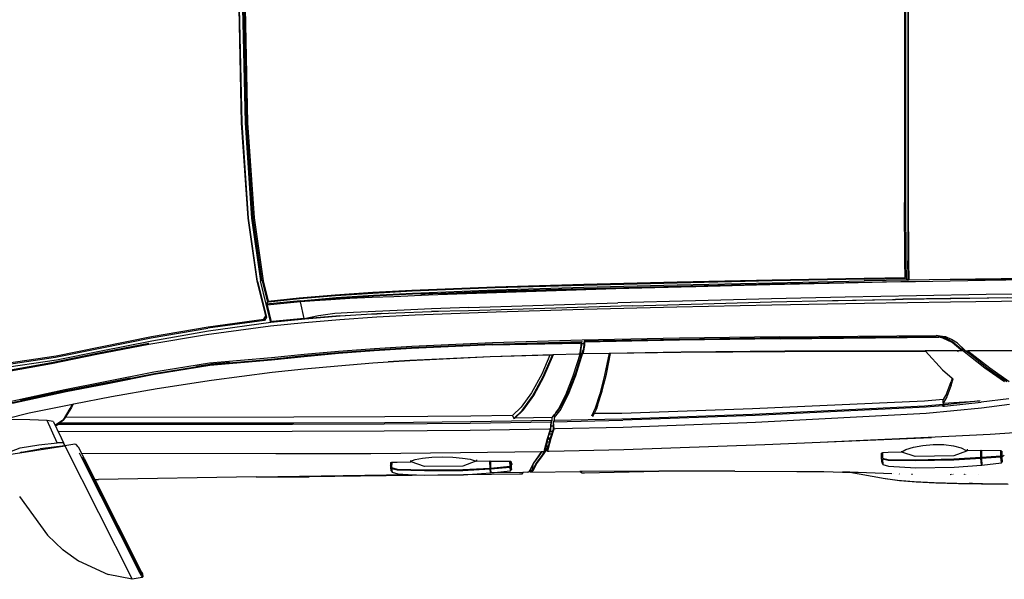
# Model space of a CAD drawing. Units: inches. Extents: x 22042254 to 25404563, y 17568978 to 17626777.
# Tile 5 of 45: x 22042255.014 to 22042256.16, y 17568977.553 to 17568978.204. Entities that reach past the tile are written whole.
import ezdxf

# ---------------------------------------------------------------- set-up
doc = ezdxf.new("R2010")
doc.units = ezdxf.units.IN
doc.header["$MEASUREMENT"] = 0
doc.layers.add('A-SITE-VEHI', color=8, linetype='Continuous', lineweight=18)
doc.layers.add('Edges', color=250, linetype='Continuous')

# ---------------------------------------------------------------- blocks, each defined once
blk = doc.blocks.new('Nissan Qashqai pl')
at = {"layer": 'Edges'}
for p, q in [((8.8918, 12.7444), (9.0186, 12.9956)), ((9.0186, 12.9956), (8.9731, 12.9865)), ((9.0374, 12.9925), (9.0186, 12.9956)), ((8.9173, 12.961), (8.9731, 12.9865)), ((9.0333, 12.9845), (8.9232, 12.7662)), ((9.0386, 12.9907), (8.9254, 12.7664)), ((8.9483, 12.8082), (9.0343, 12.9785)), ((9.0356, 12.9888), (9.0333, 12.9845)), ((9.0343, 12.9785), (9.0347, 12.9794)), ((9.0347, 12.9794), (9.0362, 12.9822)), ((9.0356, 12.9888), (9.0374, 12.9925)), ((9.0362, 12.9822), (9.037, 12.9838)), ((9.0371, 12.9841), (9.037, 12.9838)), ((9.0371, 12.9841), (9.0376, 12.985)), ((9.0376, 12.985), (9.0371, 12.9847)), ((9.0386, 12.9907), (9.0374, 12.9925)), ((9.0376, 12.985), (9.0386, 12.9907)), ((8.8885, 12.9405), (8.9173, 12.961)), ((8.8591, 12.9127), (8.8879, 12.94)), ((8.8885, 12.9405), (8.8879, 12.94)), ((8.8066, 12.84), (8.8591, 12.9127)), ((10.4573, 12.8093), (10.4889, 12.8119)), ((10.4613, 12.8099), (10.4926, 12.8125)), ((10.4889, 12.8119), (10.526, 12.8138)), ((10.4926, 12.8125), (10.5294, 12.8143)), ((10.526, 12.8138), (10.569, 12.8151)), ((10.5294, 12.8143), (10.5719, 12.8156)), ((10.569, 12.8151), (10.5919, 12.8155)), ((10.5719, 12.8156), (10.6176, 12.8164)), ((10.5919, 12.8155), (10.6151, 12.8159)), ((10.5981, 12.8157), (10.5919, 12.8155)), ((10.6174, 12.816), (10.5981, 12.8157)), ((10.6151, 12.8159), (10.6644, 12.8162)), ((10.6176, 12.8164), (10.6651, 12.8167)), ((8.928, 12.7679), (8.9483, 12.8082)), ((8.9483, 12.8082), (8.9552, 12.8081)), ((9.2517, 12.8031), (8.9552, 12.8081)), ((9.2517, 12.8031), (9.351, 12.803)), ((9.2517, 12.8031), (9.5372, 12.7983)), ((9.641, 12.7991), (9.351, 12.803)), ((9.5052, 12.7918), (9.5044, 12.7856)), ((9.5052, 12.7918), (9.5069, 12.7941)), ((9.5061, 12.7878), (9.5069, 12.7941)), ((9.5069, 12.7941), (9.5176, 12.7972)), ((9.5679, 12.792), (9.5168, 12.7904)), ((9.5176, 12.7972), (9.5372, 12.7983)), ((9.5372, 12.7983), (9.5689, 12.7999)), ((9.6401, 12.7914), (9.5679, 12.792)), ((9.5689, 12.7999), (9.641, 12.7991)), ((9.641, 12.7991), (9.6921, 12.7956)), ((9.7466, 12.7978), (9.641, 12.7991)), ((9.692, 12.7943), (9.6913, 12.7886)), ((9.6921, 12.7956), (9.692, 12.7943)), ((9.6922, 12.7943), (9.692, 12.7943)), ((9.6922, 12.7943), (9.6921, 12.7956)), ((9.7526, 12.7946), (9.6921, 12.7956)), ((9.6922, 12.7885), (9.693, 12.7955)), ((9.6922, 12.7885), (9.6922, 12.7943)), ((9.693, 12.7955), (9.7296, 12.7914)), ((9.7511, 12.7979), (9.7466, 12.7978)), ((9.7526, 12.7946), (9.7511, 12.7979)), ((9.7623, 12.7945), (9.7526, 12.7946)), ((9.7623, 12.7945), (9.7643, 12.7937)), ((9.7643, 12.7937), (9.7652, 12.7927)), ((9.7643, 12.7937), (9.7648, 12.7929)), ((9.7648, 12.7929), (9.7648, 12.7929)), ((9.7648, 12.7929), (9.7664, 12.7902)), ((9.7652, 12.7927), (9.7665, 12.7907)), ((9.7667, 12.7933), (9.7665, 12.7907)), ((9.7677, 12.7944), (9.7667, 12.7933)), ((9.7676, 12.7931), (9.7667, 12.7933)), ((9.7673, 12.7899), (9.7676, 12.7931)), ((9.769, 12.7926), (9.7676, 12.7931)), ((9.7677, 12.7944), (9.7677, 12.7944)), ((9.77, 12.7936), (9.7677, 12.7944)), ((9.7677, 12.7944), (9.8598, 12.7928)), ((9.7712, 12.7892), (9.769, 12.7926)), ((9.7734, 12.7884), (9.77, 12.7936)), ((9.8598, 12.7928), (9.8614, 12.7937)), ((9.8643, 12.7927), (9.8598, 12.7928)), ((9.8614, 12.7937), (9.8647, 12.7956)), ((10.0085, 12.7922), (9.8643, 12.7927)), ((9.8647, 12.7956), (9.869, 12.7954)), ((9.869, 12.7954), (10.0085, 12.7922)), ((10.0124, 12.7922), (10.0085, 12.7922)), ((10.1513, 12.7924), (10.0124, 12.7922)), ((10.1513, 12.7924), (10.2677, 12.793)), ((10.2677, 12.793), (10.3189, 12.7931)), ((10.3189, 12.7931), (10.3537, 12.7939)), ((10.3537, 12.7939), (10.3832, 12.7945)), ((10.3679, 12.7944), (10.3537, 12.7939)), ((10.3679, 12.7944), (10.4275, 12.8051)), ((10.4468, 12.7976), (10.3679, 12.7944)), ((10.4275, 12.8051), (10.4304, 12.8056)), ((10.4304, 12.8056), (10.4339, 12.8061)), ((10.4339, 12.8061), (10.4573, 12.8093)), ((10.4339, 12.8061), (10.4345, 12.8062)), ((10.4345, 12.8062), (10.4613, 12.8099)), ((10.4503, 12.7976), (10.4502, 12.7976)), ((10.4603, 12.7976), (10.4613, 12.7978)), ((10.4838, 12.7977), (10.4852, 12.7982)), ((10.5565, 12.7985), (10.5591, 12.7977)), ((10.5615, 12.7978), (10.5617, 12.7985)), ((10.583, 12.7984), (10.5834, 12.798)), ((10.5836, 12.798), (10.5831, 12.7984)), ((10.5847, 12.798), (10.5841, 12.7984)), ((10.5873, 12.7981), (10.5873, 12.7981)), ((10.6087, 12.7983), (10.6087, 12.7984)), ((9.5037, 12.7806), (9.5045, 12.7814)), ((9.5044, 12.7856), (9.5045, 12.7814)), ((9.5045, 12.7814), (9.5045, 12.7759)), ((9.5045, 12.7759), (9.5063, 12.7755)), ((9.5168, 12.7904), (9.5061, 12.7878)), ((9.5061, 12.7856), (9.5167, 12.7883)), ((9.5063, 12.7755), (9.5061, 12.7856)), ((9.5063, 12.7755), (9.5168, 12.7751)), ((9.5167, 12.7883), (9.5679, 12.7899)), ((9.5168, 12.7751), (9.5423, 12.7746)), ((9.5423, 12.7746), (9.5422, 12.7736)), ((9.5422, 12.7736), (9.5422, 12.7725)), ((9.5422, 12.7736), (9.5424, 12.7735)), ((9.5426, 12.7747), (9.5423, 12.7746)), ((9.5426, 12.7747), (9.5424, 12.7735)), ((9.5424, 12.7735), (9.5503, 12.7706)), ((9.5678, 12.7837), (9.5426, 12.7747)), ((9.64, 12.7831), (9.5678, 12.7837)), ((9.5679, 12.7899), (9.64, 12.7892)), ((9.64, 12.7892), (9.6912, 12.7865)), ((9.6645, 12.7737), (9.64, 12.7831)), ((9.6913, 12.7886), (9.6401, 12.7914)), ((9.6633, 12.7726), (9.6645, 12.7737)), ((9.6655, 12.7733), (9.6645, 12.7737)), ((9.6655, 12.7733), (9.6911, 12.7732)), ((9.6655, 12.7713), (9.6655, 12.7733)), ((9.6912, 12.7811), (9.6911, 12.7796)), ((9.6911, 12.7796), (9.6911, 12.7732)), ((9.6913, 12.7886), (9.6912, 12.7865)), ((9.6912, 12.7865), (9.6912, 12.7811)), ((9.692, 12.7811), (9.6912, 12.7811)), ((9.692, 12.7811), (9.6921, 12.7864)), ((9.692, 12.7796), (9.692, 12.7811)), ((9.692, 12.7733), (9.692, 12.7796)), ((9.692, 12.7733), (9.7287, 12.7734)), ((9.6922, 12.7885), (9.6921, 12.7864)), ((9.6921, 12.7864), (9.7288, 12.7832)), ((9.7288, 12.7854), (9.6922, 12.7885)), ((9.7288, 12.7832), (9.7287, 12.7734)), ((9.7287, 12.7734), (9.7305, 12.7738)), ((9.7296, 12.7914), (9.7288, 12.7854)), ((9.7306, 12.7834), (9.7288, 12.7854)), ((9.7288, 12.7854), (9.7288, 12.7832)), ((9.7288, 12.7832), (9.7306, 12.7834)), ((9.7296, 12.7914), (9.7314, 12.7895)), ((9.7305, 12.7738), (9.7306, 12.7834)), ((9.7305, 12.7738), (9.7313, 12.7798)), ((9.7306, 12.7834), (9.7314, 12.7895)), ((9.7314, 12.7895), (9.7313, 12.7798)), ((9.733, 12.7782), (9.7313, 12.7798)), ((9.7665, 12.7904), (9.7664, 12.7902)), ((9.7664, 12.7902), (9.7674, 12.7885)), ((9.7665, 12.7907), (9.7676, 12.7889)), ((9.7673, 12.7897), (9.7673, 12.7899)), ((9.7673, 12.7897), (9.7676, 12.7889)), ((9.7674, 12.7885), (9.7728, 12.7781)), ((9.7676, 12.7889), (9.7684, 12.7875)), ((9.7676, 12.7887), (9.7678, 12.7882)), ((9.7684, 12.7875), (9.7717, 12.781)), ((9.7707, 12.7848), (9.7709, 12.7893)), ((9.7717, 12.781), (9.7707, 12.7848)), ((9.7709, 12.7893), (9.7712, 12.7892)), ((9.7724, 12.7874), (9.7712, 12.7892)), ((9.7717, 12.781), (9.7738, 12.7771)), ((9.7778, 12.777), (9.7724, 12.7874)), ((9.7728, 12.7781), (9.7832, 12.7637)), ((9.7788, 12.778), (9.7734, 12.7884)), ((9.7738, 12.7771), (9.7842, 12.7627)), ((9.7883, 12.7626), (9.7778, 12.777)), ((9.7894, 12.7636), (9.7788, 12.778)), ((10.4282, 12.7775), (10.4274, 12.7679)), ((10.4282, 12.7775), (10.4299, 12.7798)), ((10.4291, 12.77), (10.4299, 12.7798)), ((10.4299, 12.7798), (10.4406, 12.7829)), ((10.4406, 12.7829), (10.4919, 12.7858)), ((10.4919, 12.7858), (10.564, 12.7851)), ((10.564, 12.7851), (10.6151, 12.7813)), ((10.615, 12.7803), (10.6142, 12.7686)), ((10.6151, 12.7813), (10.615, 12.7803)), ((10.615, 12.7676), (10.6151, 12.7803)), ((10.6151, 12.7803), (10.615, 12.7803)), ((10.6151, 12.7803), (10.6151, 12.7813)), ((10.6151, 12.7685), (10.616, 12.7812)), ((10.616, 12.7812), (10.6526, 12.7768)), ((10.6526, 12.7768), (10.6518, 12.7657)), ((10.6526, 12.7768), (10.6543, 12.7749)), ((10.6537, 12.7658), (10.6543, 12.7749)), ((10.6543, 12.7749), (10.6543, 12.7656)), ((8.7858, 12.7613), (8.807, 12.758)), ((8.8102, 12.7568), (8.807, 12.758)), ((8.807, 12.758), (8.8918, 12.7444)), ((8.8102, 12.7568), (8.8455, 12.7506)), ((8.9171, 12.7464), (8.9233, 12.7586)), ((8.9232, 12.7662), (8.9194, 12.7588)), ((8.925, 12.762), (8.9233, 12.7586)), ((8.9233, 12.7586), (9.2886, 12.7594)), ((8.928, 12.7679), (8.925, 12.762)), ((9.2886, 12.7594), (9.4673, 12.7589)), ((9.4673, 12.7589), (9.6358, 12.7575)), ((9.5503, 12.7706), (9.5641, 12.7681)), ((9.5641, 12.7681), (9.5818, 12.766)), ((9.5818, 12.766), (9.6016, 12.7651)), ((9.6016, 12.7651), (9.6215, 12.766)), ((9.6215, 12.766), (9.6395, 12.7676)), ((9.6358, 12.7575), (9.7887, 12.7552)), ((9.6395, 12.7676), (9.654, 12.7697)), ((9.654, 12.7697), (9.6633, 12.7726)), ((9.6911, 12.7732), (9.692, 12.7733)), ((9.7832, 12.7637), (9.7887, 12.7552)), ((9.7842, 12.7627), (9.7891, 12.7552)), ((9.7933, 12.7549), (9.7883, 12.7626)), ((9.7887, 12.7552), (9.7891, 12.7552)), ((9.7891, 12.7552), (9.79, 12.7552)), ((9.7965, 12.7526), (9.7894, 12.7636)), ((9.79, 12.7552), (9.7931, 12.7552)), ((9.7931, 12.7552), (9.7934, 12.7535)), ((9.7931, 12.7552), (9.7933, 12.7549)), ((9.7933, 12.7549), (9.7941, 12.7541)), ((9.7993, 12.755), (9.7986, 12.7544)), ((9.7999, 12.7522), (9.7993, 12.755)), ((9.7993, 12.755), (9.8024, 12.7549)), ((9.8024, 12.7549), (9.9426, 12.7518)), ((10.4263, 12.7665), (10.4274, 12.7674)), ((10.4274, 12.7679), (10.4274, 12.7674)), ((10.4274, 12.7674), (10.4275, 12.7586)), ((10.4293, 12.7579), (10.4275, 12.7586)), ((10.4398, 12.7724), (10.4291, 12.77)), ((10.4291, 12.7677), (10.4398, 12.7701)), ((10.4293, 12.7579), (10.4291, 12.7677)), ((10.4398, 12.7573), (10.4293, 12.7579)), ((10.4909, 12.773), (10.4398, 12.7724)), ((10.4398, 12.7701), (10.4909, 12.7708)), ((10.4653, 12.7564), (10.4398, 12.7573)), ((10.4653, 12.7561), (10.4652, 12.7545)), ((10.4908, 12.7648), (10.4653, 12.7564)), ((10.4653, 12.7564), (10.4653, 12.7561)), ((10.4653, 12.7564), (10.4653, 12.7564)), ((10.4653, 12.7564), (10.4653, 12.7561)), ((10.4653, 12.7561), (10.4653, 12.7561)), ((10.4653, 12.7561), (10.4732, 12.7517)), ((10.563, 12.7633), (10.4908, 12.7648)), ((10.5631, 12.7715), (10.4909, 12.773)), ((10.4909, 12.7708), (10.563, 12.7692)), ((10.563, 12.7692), (10.6142, 12.7663)), ((10.5867, 12.7545), (10.563, 12.7633)), ((10.6142, 12.7686), (10.5631, 12.7715)), ((10.6142, 12.766), (10.6141, 12.7537)), ((10.6142, 12.7686), (10.6142, 12.7677)), ((10.6142, 12.7677), (10.615, 12.7676)), ((10.6142, 12.7677), (10.6142, 12.7663)), ((10.6142, 12.7663), (10.6142, 12.766)), ((10.6151, 12.7676), (10.615, 12.7676)), ((10.615, 12.7537), (10.6151, 12.7659)), ((10.6518, 12.7657), (10.6151, 12.7685)), ((10.6151, 12.7676), (10.6151, 12.7685)), ((10.6151, 12.7662), (10.6151, 12.7676)), ((10.6151, 12.7662), (10.6518, 12.7634)), ((10.6151, 12.7659), (10.6151, 12.7662)), ((10.6518, 12.7634), (10.6517, 12.754)), ((10.6536, 12.7639), (10.6518, 12.7657)), ((10.6518, 12.7657), (10.6518, 12.7634)), ((10.6518, 12.7634), (10.6536, 12.7639)), ((10.6543, 12.7656), (10.6535, 12.7546)), ((10.6535, 12.7546), (10.6536, 12.7639)), ((10.6536, 12.7639), (10.6537, 12.7658)), ((10.6537, 12.7658), (10.6543, 12.7656)), ((10.6578, 12.7628), (10.6543, 12.7656)), ((8.7917, 12.7547), (8.8075, 12.7486)), ((8.8075, 12.7486), (8.8429, 12.7426)), ((8.8429, 12.7426), (8.8771, 12.7388)), ((8.8918, 12.7444), (8.8455, 12.7506)), ((8.8771, 12.7388), (8.8585, 12.6969)), ((8.8895, 12.7393), (8.8771, 12.7388)), ((8.8815, 12.7228), (8.892, 12.7444)), ((8.8815, 12.7228), (8.8895, 12.7393)), ((8.8908, 12.7421), (8.8895, 12.7393)), ((8.8906, 12.7418), (8.8895, 12.7393)), ((8.8906, 12.7418), (8.8911, 12.7428)), ((8.892, 12.7444), (8.8908, 12.7421)), ((8.8911, 12.7428), (8.8919, 12.7444)), ((8.8911, 12.7428), (8.8919, 12.7444)), ((8.8919, 12.7444), (8.8911, 12.7428)), ((8.8919, 12.7444), (8.8918, 12.7444)), ((8.892, 12.7444), (8.8919, 12.7444)), ((8.8919, 12.7444), (8.8919, 12.7444)), ((8.8919, 12.7444), (8.8919, 12.7444)), ((8.9106, 12.7413), (8.892, 12.7444)), ((8.892, 12.7444), (8.892, 12.7444)), ((8.9131, 12.7421), (8.9106, 12.7413)), ((8.9171, 12.7464), (8.9131, 12.7421)), ((8.9171, 12.7464), (8.917, 12.7468)), ((9.7934, 12.7535), (9.7938, 12.7538)), ((9.7934, 12.7535), (9.7937, 12.7524)), ((9.7937, 12.7524), (9.7992, 12.7308)), ((9.7941, 12.7541), (9.7943, 12.7535)), ((9.7955, 12.7516), (9.7943, 12.7535)), ((9.7943, 12.7535), (9.7964, 12.7453)), ((9.7963, 12.7523), (9.7955, 12.7516)), ((9.7963, 12.7523), (9.7963, 12.7524)), ((9.7964, 12.7524), (9.7963, 12.7523)), ((9.7992, 12.7476), (9.7963, 12.7523)), ((9.7967, 12.7526), (9.7964, 12.7524)), ((9.7964, 12.7525), (9.7964, 12.7524)), ((9.7964, 12.7524), (9.7996, 12.7475)), ((9.7964, 12.7453), (9.7992, 12.7476)), ((9.7964, 12.7453), (9.7973, 12.7418)), ((9.7983, 12.7541), (9.7965, 12.7526)), ((9.7965, 12.7526), (9.7967, 12.7526)), ((9.7977, 12.7535), (9.7967, 12.7526)), ((9.7967, 12.7526), (9.7986, 12.7526)), ((9.7977, 12.7431), (9.7973, 12.7418)), ((9.7973, 12.7418), (9.7977, 12.7409)), ((9.7973, 12.7418), (9.7977, 12.7399)), ((9.7982, 12.754), (9.7977, 12.7535)), ((9.7977, 12.7444), (9.7985, 12.7451)), ((9.7985, 12.7451), (9.7977, 12.7431)), ((9.7977, 12.7431), (9.7977, 12.7444)), ((9.7977, 12.7399), (9.7977, 12.7409)), ((9.7977, 12.7409), (9.7987, 12.7388)), ((9.7977, 12.7399), (9.7978, 12.7397)), ((9.7987, 12.7388), (9.7978, 12.7397)), ((9.7978, 12.7397), (9.7987, 12.7362)), ((9.7983, 12.7541), (9.7982, 12.754)), ((9.7986, 12.7526), (9.7982, 12.754)), ((9.7986, 12.7544), (9.7983, 12.7541)), ((9.7989, 12.7461), (9.7985, 12.7451)), ((9.7988, 12.7516), (9.7986, 12.7526)), ((9.7987, 12.7388), (9.7992, 12.7377)), ((9.7987, 12.7362), (9.7992, 12.7377)), ((9.7998, 12.7477), (9.7988, 12.7516)), ((9.7998, 12.7466), (9.7989, 12.7461)), ((9.7998, 12.7466), (9.7992, 12.7476)), ((9.7992, 12.7377), (9.8027, 12.7364)), ((9.7996, 12.7475), (9.7998, 12.7477)), ((9.8002, 12.7461), (9.7996, 12.7475)), ((9.8001, 12.7468), (9.7996, 12.7475)), ((9.8001, 12.7468), (9.7998, 12.7477)), ((9.8003, 12.7458), (9.7998, 12.7466)), ((9.8054, 12.7307), (9.7999, 12.7522)), ((9.8002, 12.7461), (9.8001, 12.7468)), ((9.8003, 12.7458), (9.8002, 12.7461)), ((9.8027, 12.7364), (9.8003, 12.7458)), ((9.8031, 12.7349), (9.8027, 12.7364)), ((9.9426, 12.7518), (10.2081, 12.7424)), ((10.2081, 12.7424), (10.312, 12.7377)), ((10.312, 12.7377), (10.5214, 12.7293)), ((10.312, 12.7377), (10.5147, 12.7285)), ((10.4732, 12.7517), (10.4871, 12.7474)), ((10.4871, 12.7474), (10.5048, 12.744)), ((10.5048, 12.744), (10.5246, 12.7423)), ((10.5246, 12.7423), (10.5445, 12.7425)), ((10.5445, 12.7425), (10.5625, 12.7446)), ((10.5625, 12.7446), (10.5769, 12.7484)), ((10.5769, 12.7484), (10.5863, 12.7537)), ((10.5863, 12.7537), (10.5867, 12.7545)), ((10.5885, 12.7538), (10.5867, 12.7545)), ((10.5885, 12.751), (10.5885, 12.7538)), ((10.6141, 12.7537), (10.5885, 12.7538)), ((10.6141, 12.7537), (10.615, 12.7537)), ((10.6517, 12.754), (10.615, 12.7537)), ((10.6535, 12.7546), (10.6517, 12.754)), ((8.8734, 12.7057), (8.8793, 12.7181)), ((8.8793, 12.7181), (8.8815, 12.7228)), ((9.3194, 12.7179), (8.8793, 12.7181)), ((9.4919, 12.7173), (9.3194, 12.7179)), ((9.7987, 12.7362), (9.8002, 12.7301)), ((9.7992, 12.7308), (9.8044, 12.7151)), ((9.8002, 12.7301), (9.8008, 12.7285)), ((9.8008, 12.7285), (9.8014, 12.7303)), ((9.8008, 12.7285), (9.8014, 12.7265)), ((9.8014, 12.7303), (9.8031, 12.7349)), ((9.8043, 12.7303), (9.8014, 12.7303)), ((9.8014, 12.7265), (9.803, 12.723)), ((9.8014, 12.7265), (9.8026, 12.723)), ((9.803, 12.723), (9.8026, 12.723)), ((9.8026, 12.723), (9.8046, 12.7171)), ((9.8067, 12.7229), (9.803, 12.723)), ((9.8043, 12.7303), (9.8031, 12.7349)), ((9.8044, 12.73), (9.8043, 12.7303)), ((9.8067, 12.7229), (9.8044, 12.73)), ((9.8106, 12.715), (9.8054, 12.7307)), ((9.8086, 12.7171), (9.8067, 12.7229)), ((10.5147, 12.7285), (10.6318, 12.7228)), ((10.6318, 12.7228), (10.6955, 12.7184)), ((8.87, 12.6987), (8.8734, 12.7057)), ((8.8734, 12.7057), (8.8768, 12.7057)), ((8.8751, 12.7054), (8.8768, 12.7057)), ((8.8893, 12.6956), (8.8751, 12.7054)), ((8.8768, 12.7057), (8.879, 12.704)), ((8.879, 12.704), (9.3198, 12.7039)), ((8.879, 12.704), (8.881, 12.7023)), ((9.3225, 12.7021), (8.881, 12.7023)), ((8.881, 12.7023), (8.8893, 12.6956)), ((9.3198, 12.7039), (9.4922, 12.7033)), ((9.4936, 12.7013), (9.3225, 12.7021)), ((9.6538, 12.7157), (9.4919, 12.7173)), ((9.4922, 12.7033), (9.654, 12.7018)), ((9.6552, 12.6997), (9.4936, 12.7013)), ((9.802, 12.7133), (9.6538, 12.7157)), ((9.654, 12.7018), (9.8061, 12.6994)), ((9.8078, 12.6971), (9.6552, 12.6997)), ((9.8051, 12.7132), (9.802, 12.7133)), ((9.8044, 12.7151), (9.8051, 12.7132)), ((9.8046, 12.7171), (9.8086, 12.7171)), ((9.8046, 12.7171), (9.8055, 12.7143)), ((9.8061, 12.6994), (9.8051, 12.7132)), ((9.8055, 12.7143), (9.8058, 12.7073)), ((9.8058, 12.7073), (9.8098, 12.7073)), ((9.8058, 12.7073), (9.8061, 12.6994)), ((9.8061, 12.6994), (9.8078, 12.6971)), ((9.8096, 12.7142), (9.8086, 12.7171)), ((9.8098, 12.7073), (9.8096, 12.7142)), ((9.8101, 12.6993), (9.8098, 12.7073)), ((9.8101, 12.6993), (9.8112, 12.7131)), ((9.8119, 12.697), (9.8101, 12.6993)), ((9.8101, 12.6993), (9.9411, 12.6966)), ((9.8112, 12.7131), (9.8106, 12.715)), ((9.8143, 12.713), (9.8112, 12.7131)), ((9.9414, 12.71), (9.8143, 12.713)), ((10.19, 12.7008), (9.9414, 12.71)), ((10.5113, 12.6839), (10.19, 12.7008)), ((8.7828, 12.6934), (8.8245, 12.6828)), ((8.8259, 12.6959), (8.7916, 12.6954)), ((8.8245, 12.6828), (8.9063, 12.6663)), ((8.8585, 12.6969), (8.8259, 12.6959)), ((8.87, 12.6987), (8.8585, 12.6969)), ((8.8893, 12.6956), (8.9021, 12.6745)), ((8.8913, 12.6936), (8.8893, 12.6956)), ((8.8927, 12.6913), (8.8913, 12.6936)), ((9.3224, 12.6911), (8.8927, 12.6913)), ((8.9041, 12.6725), (8.8927, 12.6913)), ((9.3225, 12.6911), (9.3224, 12.6911)), ((9.4936, 12.6904), (9.3225, 12.6911)), ((9.6552, 12.6888), (9.4936, 12.6904)), ((9.7337, 12.6875), (9.6552, 12.6888)), ((9.7337, 12.6875), (9.7357, 12.6935)), ((9.7499, 12.6721), (9.7337, 12.6875)), ((9.7357, 12.6935), (9.7378, 12.6924)), ((9.7357, 12.6935), (9.7519, 12.678)), ((9.7378, 12.6924), (9.754, 12.677)), ((9.8078, 12.6913), (9.7378, 12.6924)), ((9.8078, 12.6971), (9.8078, 12.6913)), ((9.8078, 12.6913), (9.8119, 12.6862)), ((9.9393, 12.6944), (9.8119, 12.697)), ((9.8119, 12.6912), (9.8119, 12.697)), ((9.8241, 12.6756), (9.8119, 12.6912)), ((9.8119, 12.6862), (9.8119, 12.6912)), ((9.8147, 12.6826), (9.8119, 12.6862)), ((9.8147, 12.6826), (9.8147, 12.6826)), ((9.8147, 12.6826), (9.8201, 12.6756)), ((9.8241, 12.6706), (9.8147, 12.6826)), ((9.8891, 12.6741), (9.8818, 12.6891)), ((9.8867, 12.6842), (9.8838, 12.6901)), ((9.9393, 12.684), (9.8867, 12.6842)), ((9.8911, 12.675), (9.8867, 12.6842)), ((10.1849, 12.6857), (9.9393, 12.6944)), ((10.1849, 12.6754), (9.9393, 12.684)), ((10.1894, 12.6879), (9.9411, 12.6966)), ((10.5079, 12.6703), (10.1849, 12.6857)), ((10.5109, 12.6721), (10.1894, 12.6879)), ((10.6152, 12.674), (10.5113, 12.6839)), ((8.8941, 12.6418), (8.7925, 12.664)), ((8.8942, 12.6432), (8.7931, 12.6653)), ((8.9021, 12.6745), (8.9063, 12.6663)), ((8.9075, 12.6661), (8.9041, 12.6725)), ((8.9063, 12.6663), (8.9075, 12.6661)), ((8.9075, 12.6661), (8.9087, 12.6658)), ((8.9087, 12.6658), (8.9797, 12.6518)), ((9.7692, 12.6453), (9.7499, 12.6721)), ((9.7519, 12.678), (9.7713, 12.6512)), ((9.754, 12.677), (9.7733, 12.6502)), ((9.8201, 12.6756), (9.8338, 12.6486)), ((9.8378, 12.6485), (9.8241, 12.6756)), ((9.8378, 12.6435), (9.8241, 12.6706)), ((9.8978, 12.6472), (9.8891, 12.6741)), ((9.8911, 12.6749), (9.8911, 12.675)), ((9.8931, 12.6691), (9.8911, 12.6749)), ((9.8911, 12.6749), (9.8998, 12.6481)), ((9.8931, 12.669), (9.8931, 12.6691)), ((9.8931, 12.669), (9.9018, 12.6421)), ((10.5079, 12.6607), (10.1849, 12.6754)), ((10.543, 12.6671), (10.5079, 12.6703)), ((10.5417, 12.6693), (10.5109, 12.6721)), ((10.5417, 12.6693), (10.5427, 12.6702)), ((10.5417, 12.6693), (10.543, 12.6671)), ((10.5436, 12.6687), (10.5427, 12.6702)), ((10.5427, 12.6702), (10.5458, 12.67)), ((10.544, 12.6678), (10.543, 12.6671)), ((10.543, 12.6646), (10.543, 12.6671)), ((10.543, 12.6646), (10.543, 12.6576)), ((10.5439, 12.6646), (10.543, 12.6646)), ((10.5502, 12.6526), (10.543, 12.6646)), ((10.544, 12.6678), (10.5436, 12.6687)), ((10.5439, 12.6646), (10.613, 12.6601)), ((10.547, 12.6674), (10.544, 12.6678)), ((10.5458, 12.67), (10.6144, 12.6629)), ((10.613, 12.6601), (10.547, 12.6674)), ((10.6664, 12.6566), (10.6144, 12.6629)), ((10.6678, 12.6672), (10.6152, 12.674)), ((8.8918, 12.6392), (8.7881, 12.6621)), ((8.8083, 12.6591), (8.8954, 12.6403)), ((8.9797, 12.6518), (9.0656, 12.6372)), ((9.7885, 12.6099), (9.7692, 12.6453)), ((9.7713, 12.6512), (9.7905, 12.6158)), ((9.7733, 12.6502), (9.7925, 12.6148)), ((9.8338, 12.6486), (9.8475, 12.613)), ((9.8516, 12.6129), (9.8378, 12.6485)), ((9.9066, 12.6119), (9.8978, 12.6472)), ((9.9086, 12.6129), (9.8998, 12.6481)), ((10.543, 12.6576), (10.5079, 12.6607)), ((10.5502, 12.6456), (10.543, 12.6576)), ((10.5584, 12.6306), (10.5502, 12.6526)), ((10.5502, 12.6456), (10.5584, 12.6236)), ((8.9679, 12.6241), (8.8918, 12.6392)), ((9.0601, 12.6092), (8.8941, 12.6418)), ((8.9696, 12.6285), (8.8942, 12.6432)), ((8.8961, 12.6401), (8.9704, 12.6257)), ((9.06, 12.6106), (8.9696, 12.6285)), ((8.9704, 12.6257), (8.9708, 12.6256)), ((8.9708, 12.6256), (9.0143, 12.6169)), ((9.0656, 12.6372), (9.1676, 12.6212)), ((9.8516, 12.6079), (9.8378, 12.6435)), ((9.9018, 12.6421), (9.9106, 12.6068)), ((10.5584, 12.6306), (10.5617, 12.619)), ((8.8666, 12.5888), (8.7287, 12.6134)), ((8.7292, 12.6146), (8.8666, 12.5901)), ((9.0591, 12.6065), (8.9679, 12.6241)), ((9.1644, 12.5938), (9.06, 12.6106)), ((9.1645, 12.5924), (9.0601, 12.6092)), ((9.1676, 12.6212), (9.2814, 12.6065)), ((9.8039, 12.5741), (9.7885, 12.6099)), ((9.7905, 12.6158), (9.8087, 12.574)), ((9.7925, 12.6148), (9.8107, 12.573)), ((9.8475, 12.613), (9.8611, 12.5708)), ((9.8652, 12.5704), (9.8516, 12.6129)), ((9.8652, 12.5654), (9.8516, 12.6079)), ((9.9149, 12.5705), (9.9066, 12.6119)), ((9.9169, 12.5714), (9.9086, 12.6129)), ((9.9106, 12.6068), (9.9177, 12.5714)), ((10.5419, 12.6018), (10.56, 12.6176)), ((10.56, 12.6176), (10.5584, 12.6236)), ((10.56, 12.6176), (10.5617, 12.619)), ((10.6583, 12.6245), (10.6215, 12.5986)), ((10.6627, 12.6241), (10.6261, 12.5984)), ((10.6306, 12.5982), (10.6671, 12.6238)), ((8.7481, 12.5968), (8.8745, 12.5782)), ((8.7491, 12.594), (8.8754, 12.5755)), ((8.8761, 12.5839), (8.7496, 12.6025)), ((8.8666, 12.5901), (8.9521, 12.5726)), ((8.9522, 12.5713), (8.8666, 12.5888)), ((9.1639, 12.5895), (9.0591, 12.6065)), ((9.1393, 12.5951), (9.1647, 12.591)), ((9.2801, 12.5794), (9.1639, 12.5895)), ((9.2803, 12.5836), (9.1644, 12.5938)), ((9.2804, 12.5821), (9.1645, 12.5924)), ((9.1647, 12.591), (9.1668, 12.5908)), ((9.1668, 12.5908), (9.2019, 12.5877)), ((9.2814, 12.6065), (9.3416, 12.5999)), ((9.3416, 12.5999), (9.4048, 12.5941)), ((9.4048, 12.5941), (9.471, 12.5888)), ((9.471, 12.5888), (9.4997, 12.5869)), ((10.51, 12.5666), (10.5419, 12.6018)), ((10.6215, 12.5986), (10.5796, 12.5655)), ((10.5892, 12.5659), (10.6306, 12.5982)), ((10.6261, 12.5984), (10.593, 12.5726)), ((8.8745, 12.5782), (8.9583, 12.5609)), ((8.8754, 12.5755), (8.9591, 12.5583)), ((8.9598, 12.5666), (8.8761, 12.5839)), ((8.9521, 12.5726), (9.0495, 12.5536)), ((9.0497, 12.5523), (8.9522, 12.5713)), ((9.3418, 12.5729), (9.2801, 12.5794)), ((9.3418, 12.5771), (9.2803, 12.5836)), ((9.3419, 12.5756), (9.2804, 12.5821)), ((9.4062, 12.5713), (9.3418, 12.5771)), ((9.4064, 12.5671), (9.3418, 12.5729)), ((9.4063, 12.5699), (9.3419, 12.5756)), ((9.4735, 12.5663), (9.4062, 12.5713)), ((9.4736, 12.5648), (9.4063, 12.5699)), ((9.5404, 12.5844), (9.4997, 12.5869)), ((9.4997, 12.5869), (9.5403, 12.5842)), ((9.5403, 12.5842), (9.6913, 12.5767)), ((9.6912, 12.5774), (9.5404, 12.5844)), ((9.8039, 12.5741), (9.6912, 12.5774)), ((9.6913, 12.5767), (9.8099, 12.573)), ((9.8087, 12.574), (9.8039, 12.5741)), ((9.8099, 12.573), (9.8087, 12.574)), ((9.8099, 12.573), (9.8107, 12.573)), ((9.8107, 12.573), (9.8573, 12.5716)), ((9.8573, 12.5716), (9.8603, 12.5715)), ((9.8603, 12.5715), (9.8605, 12.5696)), ((9.8611, 12.5708), (9.8603, 12.5715)), ((9.8612, 12.5707), (9.8611, 12.5708)), ((9.8612, 12.5707), (9.8615, 12.5688)), ((9.8652, 12.5706), (9.8664, 12.5714)), ((9.8652, 12.5706), (9.8665, 12.5695)), ((9.8652, 12.5704), (9.8652, 12.5706)), ((9.8652, 12.5704), (9.8652, 12.5704)), ((9.8652, 12.5704), (9.8652, 12.5654)), ((9.8655, 12.5687), (9.8652, 12.5704)), ((9.8665, 12.5695), (9.8664, 12.5714)), ((9.8664, 12.5714), (9.9149, 12.5705)), ((9.9149, 12.5705), (10.0505, 12.5681)), ((9.9177, 12.5714), (9.9169, 12.5714)), ((10.0501, 12.5695), (9.9177, 12.5714)), ((10.593, 12.5726), (10.584, 12.5655)), ((8.9583, 12.5609), (9.0538, 12.5419)), ((8.9591, 12.5583), (9.0546, 12.5394)), ((9.0552, 12.5477), (8.9598, 12.5666)), ((9.0495, 12.5536), (9.1584, 12.5351)), ((9.4739, 12.5621), (9.4064, 12.5671)), ((9.5437, 12.5619), (9.4735, 12.5663)), ((9.5438, 12.5605), (9.4736, 12.5648)), ((9.5443, 12.5579), (9.4739, 12.5621)), ((9.6953, 12.5549), (9.5437, 12.5619)), ((9.6954, 12.5535), (9.5438, 12.5605)), ((9.696, 12.551), (9.5443, 12.5579)), ((9.6953, 12.5549), (9.8598, 12.5517)), ((9.6953, 12.5549), (9.863, 12.5497)), ((9.6954, 12.5535), (9.8641, 12.5483)), ((9.8629, 12.5516), (9.8598, 12.5517)), ((9.8605, 12.5696), (9.8626, 12.5564)), ((9.8615, 12.5688), (9.8635, 12.5556)), ((9.8626, 12.5564), (9.8627, 12.5532)), ((9.8637, 12.5532), (9.8627, 12.5532)), ((9.8627, 12.5532), (9.8629, 12.5516)), ((9.8629, 12.5516), (9.863, 12.5497)), ((9.8635, 12.5556), (9.8637, 12.5532)), ((9.8643, 12.5532), (9.8637, 12.5532)), ((9.8637, 12.5532), (9.8638, 12.5508)), ((9.8677, 12.5531), (9.8643, 12.5532)), ((9.8675, 12.5555), (9.8655, 12.5687)), ((9.8686, 12.5562), (9.8665, 12.5695)), ((9.8677, 12.5531), (9.8675, 12.5555)), ((9.8678, 12.5507), (9.8677, 12.5531)), ((9.8689, 12.5515), (9.8686, 12.5562)), ((9.869, 12.5496), (9.8689, 12.5515)), ((10.2453, 12.568), (10.0501, 12.5695)), ((10.0505, 12.5681), (10.2453, 12.5664)), ((10.4292, 12.5674), (10.2453, 12.568)), ((10.2453, 12.5664), (10.4289, 12.5658)), ((10.4289, 12.5658), (10.5092, 12.5658)), ((10.5099, 12.5674), (10.4292, 12.5674)), ((10.5099, 12.5674), (10.5092, 12.5658)), ((10.5092, 12.5658), (10.5094, 12.5658)), ((10.5094, 12.5658), (10.51, 12.5666)), ((10.5783, 12.5659), (10.5094, 12.5658)), ((10.51, 12.5666), (10.5099, 12.5674)), ((10.57, 12.5517), (10.5589, 12.5451)), ((10.5764, 12.5642), (10.5598, 12.5507)), ((10.5776, 12.5633), (10.5612, 12.5498)), ((10.5834, 12.5641), (10.57, 12.5517)), ((10.57, 12.5517), (10.5821, 12.5633)), ((10.5709, 12.5675), (10.5705, 12.5671)), ((10.5719, 12.5682), (10.5709, 12.5675)), ((10.5783, 12.5659), (10.5764, 12.5642)), ((10.5776, 12.5633), (10.5783, 12.5659)), ((10.5796, 12.5655), (10.5776, 12.5633)), ((10.5796, 12.5655), (10.5783, 12.5659)), ((10.5796, 12.562), (10.5796, 12.5655)), ((10.5838, 12.5653), (10.5821, 12.5633)), ((10.584, 12.5647), (10.5834, 12.5641)), ((10.584, 12.5655), (10.5838, 12.5653)), ((10.584, 12.5655), (10.5841, 12.5655)), ((10.584, 12.5654), (10.584, 12.5655)), ((10.5847, 12.5655), (10.584, 12.5647)), ((10.584, 12.5647), (10.584, 12.5654)), ((10.5851, 12.5659), (10.5841, 12.5655)), ((10.5841, 12.5655), (10.5847, 12.5655)), ((10.5851, 12.5659), (10.5847, 12.5655)), ((10.5851, 12.5659), (10.5892, 12.5659)), ((10.6988, 12.5662), (10.5892, 12.5659)), ((9.0538, 12.5419), (9.1605, 12.5233)), ((9.0546, 12.5394), (9.1612, 12.5208)), ((9.1617, 12.5292), (9.0552, 12.5477)), ((9.1584, 12.5351), (9.2783, 12.5191)), ((9.8644, 12.5459), (9.696, 12.551)), ((9.8641, 12.5483), (9.863, 12.5497)), ((9.8638, 12.5508), (9.8641, 12.5483)), ((10.0472, 12.5423), (9.8644, 12.5459)), ((9.8681, 12.5482), (9.8678, 12.5507)), ((9.8681, 12.5482), (9.869, 12.5496)), ((10.0476, 12.5445), (9.8681, 12.5482)), ((10.0477, 12.5459), (9.869, 12.5496)), ((10.2357, 12.5398), (10.0472, 12.5423)), ((10.2367, 12.5419), (10.0476, 12.5445)), ((10.2369, 12.5433), (10.0477, 12.5459)), ((10.2357, 12.5398), (10.53, 12.5373)), ((10.2367, 12.5419), (10.5351, 12.5392)), ((10.2369, 12.5433), (10.5348, 12.5406)), ((10.4153, 12.5384), (10.4176, 12.5384)), ((10.4176, 12.5384), (10.4181, 12.5384)), ((10.4181, 12.5384), (10.4552, 12.538)), ((10.4181, 12.5384), (10.4181, 12.5384)), ((10.4778, 12.5378), (10.53, 12.5373)), ((10.5301, 12.5373), (10.53, 12.5373)), ((10.5335, 12.5378), (10.5301, 12.5373)), ((10.5419, 12.5391), (10.5335, 12.5378)), ((10.5422, 12.542), (10.5348, 12.5406)), ((10.5418, 12.5405), (10.5351, 12.5392)), ((10.5424, 12.5406), (10.5418, 12.5405)), ((10.5419, 12.5391), (10.5463, 12.541)), ((10.5479, 12.54), (10.5419, 12.5391)), ((10.5522, 12.5465), (10.5422, 12.542)), ((10.5495, 12.5438), (10.5424, 12.5406)), ((10.5463, 12.541), (10.5551, 12.5457)), ((10.5589, 12.5451), (10.5479, 12.54)), ((10.5546, 12.546), (10.5495, 12.5438)), ((10.5598, 12.5507), (10.5522, 12.5465)), ((10.5583, 12.5481), (10.5546, 12.546)), ((10.5551, 12.5457), (10.5583, 12.5481)), ((10.5612, 12.5498), (10.5583, 12.5481)), ((9.2669, 12.5088), (9.1605, 12.5233)), ((9.1612, 12.5208), (9.2656, 12.5065)), ((9.2789, 12.5131), (9.1617, 12.5292)), ((9.2783, 12.5191), (9.3422, 12.5126)), ((9.2694, 12.5006), (9.2535, 12.4354)), ((9.2543, 12.4356), (9.2707, 12.5028)), ((9.2656, 12.5065), (9.2669, 12.5088)), ((9.2656, 12.5065), (9.2694, 12.5006)), ((9.2707, 12.5028), (9.2669, 12.5088)), ((9.2707, 12.5028), (9.2694, 12.5006)), ((9.2789, 12.5131), (9.2704, 12.4783)), ((9.2724, 12.4804), (9.2799, 12.5114)), ((9.2799, 12.5114), (9.2789, 12.5131)), ((9.3427, 12.5066), (9.2789, 12.5131)), ((9.2819, 12.5112), (9.2799, 12.5114)), ((9.2803, 12.5116), (9.2822, 12.5118)), ((9.3418, 12.5051), (9.2819, 12.5112)), ((9.3418, 12.5051), (9.3346, 12.4741)), ((9.342, 12.5059), (9.3418, 12.5051)), ((9.3687, 12.5), (9.342, 12.5059)), ((9.4087, 12.5003), (9.342, 12.5059)), ((9.3422, 12.5126), (9.4088, 12.507)), ((9.4093, 12.5011), (9.3427, 12.5066)), ((9.3992, 12.496), (9.3687, 12.5)), ((9.4347, 12.494), (9.3992, 12.496)), ((9.4087, 12.5003), (9.4688, 12.4968)), ((9.4088, 12.507), (9.4782, 12.5024)), ((9.4785, 12.4965), (9.4093, 12.5011)), ((9.4688, 12.4968), (9.4789, 12.4964)), ((9.4782, 12.5024), (9.5503, 12.4987)), ((9.4789, 12.4964), (9.4785, 12.4965)), ((9.4862, 12.4961), (9.4785, 12.4965)), ((9.4789, 12.4964), (9.4862, 12.4961)), ((9.4862, 12.4961), (9.514, 12.4949)), ((9.5503, 12.4987), (9.7029, 12.4926)), ((9.2704, 12.4783), (9.2598, 12.4348)), ((9.2724, 12.4804), (9.2704, 12.4783)), ((9.2726, 12.4746), (9.2704, 12.4783)), ((9.3346, 12.4718), (9.2704, 12.4783)), ((9.3346, 12.4741), (9.2724, 12.4804)), ((9.4761, 12.4919), (9.4347, 12.494)), ((9.5168, 12.4903), (9.4761, 12.4919)), ((9.514, 12.4949), (9.5811, 12.492)), ((9.5812, 12.4874), (9.5168, 12.4903)), ((9.651, 12.4906), (9.5811, 12.492)), ((9.5811, 12.492), (9.594, 12.4914)), ((9.6514, 12.4849), (9.5812, 12.4874)), ((9.9583, 12.4812), (9.651, 12.4906)), ((9.6514, 12.4849), (9.9312, 12.4761)), ((9.7029, 12.4926), (9.8673, 12.4878)), ((9.8673, 12.4878), (10.0423, 12.4835)), ((9.9583, 12.4812), (10.091, 12.4775)), ((10.0423, 12.4835), (10.2211, 12.4795)), ((10.091, 12.4775), (10.2202, 12.4743)), ((10.2211, 12.4795), (10.3955, 12.4762)), ((9.2629, 12.435), (9.2726, 12.4746)), ((9.2649, 12.4348), (9.2741, 12.4725)), ((9.2746, 12.4744), (9.2726, 12.4746)), ((9.2741, 12.4725), (9.3326, 12.4666)), ((9.333, 12.4685), (9.2746, 12.4744)), ((9.3326, 12.4666), (9.4, 12.4609)), ((9.4004, 12.4629), (9.333, 12.4685)), ((9.3346, 12.4741), (9.3344, 12.4733)), ((9.3344, 12.4733), (9.4017, 12.4677)), ((9.3344, 12.4733), (9.3611, 12.4715)), ((9.3346, 12.4718), (9.4018, 12.4661)), ((9.3611, 12.4715), (9.3918, 12.4695)), ((9.3918, 12.4695), (9.4276, 12.4674)), ((9.4, 12.4609), (9.4706, 12.4561)), ((9.4709, 12.4581), (9.4004, 12.4629)), ((9.4017, 12.4677), (9.472, 12.463)), ((9.4018, 12.4661), (9.472, 12.4614)), ((9.4276, 12.4674), (9.4694, 12.4654)), ((9.4694, 12.4654), (9.5105, 12.4637)), ((9.472, 12.463), (9.5454, 12.4591)), ((9.472, 12.4614), (9.5454, 12.4576)), ((9.5105, 12.4637), (9.5755, 12.4608)), ((9.5454, 12.4591), (9.5454, 12.4593)), ((9.5695, 12.4589), (9.5454, 12.4591)), ((9.5609, 12.4593), (9.5695, 12.4589)), ((9.5786, 12.4588), (9.5695, 12.4589)), ((9.5695, 12.4589), (9.7014, 12.4536)), ((9.5755, 12.4608), (9.6472, 12.4581)), ((9.6206, 12.4581), (9.5786, 12.4588)), ((10.0776, 12.4719), (9.9312, 12.4761)), ((10.2201, 12.4683), (10.0776, 12.4719)), ((10.3586, 12.4651), (10.2201, 12.4683)), ((10.2202, 12.4743), (10.2203, 12.4743)), ((10.2203, 12.4743), (10.3353, 12.4717)), ((10.3353, 12.4717), (10.4477, 12.4694)), ((10.3353, 12.4717), (10.346, 12.4714)), ((10.346, 12.4714), (10.4477, 12.4694)), ((10.4931, 12.4624), (10.3586, 12.4651)), ((10.3955, 12.4762), (10.5572, 12.4737)), ((10.4477, 12.4694), (10.4538, 12.4693)), ((10.4538, 12.4693), (10.4681, 12.469)), ((10.4676, 12.4691), (10.4538, 12.4693)), ((10.5566, 12.4677), (10.4676, 12.4691)), ((10.4676, 12.4691), (10.546, 12.4677)), ((10.4681, 12.469), (10.5866, 12.467)), ((10.6237, 12.4603), (10.4931, 12.4624)), ((10.546, 12.4677), (10.546, 12.4678)), ((10.546, 12.4677), (10.5576, 12.4675)), ((10.7, 12.4662), (10.5566, 12.4677)), ((10.5572, 12.4737), (10.7004, 12.4722)), ((10.5576, 12.4675), (10.6649, 12.4659)), ((10.5866, 12.467), (10.6649, 12.4659)), ((10.7502, 12.4586), (10.6237, 12.4603)), ((9.4706, 12.4561), (9.5443, 12.4522)), ((9.5446, 12.4542), (9.4709, 12.4581)), ((9.5443, 12.4522), (9.701, 12.4459)), ((9.7011, 12.4478), (9.5446, 12.4542)), ((9.5454, 12.4576), (9.7014, 12.4513)), ((9.6714, 12.4567), (9.6206, 12.4581)), ((9.6414, 12.458), (9.6407, 12.458)), ((9.6472, 12.4581), (9.9278, 12.4492)), ((9.6549, 12.4576), (9.6558, 12.4574)), ((9.6825, 12.4564), (9.6714, 12.4567)), ((9.6825, 12.4564), (9.6829, 12.4563)), ((9.6943, 12.456), (9.6825, 12.4564)), ((9.6943, 12.4558), (9.6943, 12.456)), ((9.6951, 12.456), (9.6943, 12.456)), ((9.6951, 12.4558), (9.6951, 12.456)), ((9.8565, 12.451), (9.6951, 12.456)), ((9.701, 12.4459), (9.8673, 12.441)), ((9.8673, 12.443), (9.7011, 12.4478)), ((9.7014, 12.4536), (9.8673, 12.4488)), ((9.7014, 12.4513), (9.8673, 12.4464)), ((9.9794, 12.4475), (9.8565, 12.451)), ((9.8673, 12.4488), (10.0429, 12.4444)), ((9.8673, 12.4464), (10.0429, 12.4421)), ((10.043, 12.4387), (9.8673, 12.443)), ((9.8673, 12.441), (10.0431, 12.4367)), ((9.9278, 12.4492), (10.0747, 12.445)), ((10.0998, 12.4443), (9.9794, 12.4475)), ((10.0429, 12.4444), (10.2216, 12.4404)), ((10.0429, 12.4421), (10.2215, 12.4381)), ((10.0747, 12.445), (10.078, 12.4449)), ((10.078, 12.4449), (10.2146, 12.4414)), ((10.2146, 12.4414), (10.0998, 12.4443)), ((10.2146, 12.4414), (10.2175, 12.4413)), ((10.2175, 12.4413), (10.3564, 12.4382)), ((10.2216, 12.4404), (10.3947, 12.4371)), ((9.2535, 12.4354), (9.2362, 12.3167)), ((9.2543, 12.4356), (9.2371, 12.3169)), ((9.2426, 12.3164), (9.2598, 12.4348)), ((9.2629, 12.435), (9.2457, 12.3164)), ((9.2476, 12.3163), (9.2649, 12.4348)), ((10.2218, 12.4347), (10.043, 12.4387)), ((10.0431, 12.4367), (10.2218, 12.4327)), ((10.2215, 12.4381), (10.3945, 12.4348)), ((10.3947, 12.4314), (10.2218, 12.4347)), ((10.2218, 12.4327), (10.3947, 12.4294)), ((10.3564, 12.4382), (10.4638, 12.436)), ((10.4773, 12.4335), (10.3945, 12.4348)), ((10.3947, 12.4371), (10.4638, 12.436)), ((10.3947, 12.4314), (10.4735, 12.4301)), ((10.3947, 12.4294), (10.4715, 12.4282)), ((10.4638, 12.436), (10.4914, 12.4355)), ((10.4715, 12.4282), (10.4711, 12.3973)), ((10.4731, 12.3973), (10.4735, 12.4301)), ((10.4735, 12.4301), (10.4773, 12.4335)), ((10.4773, 12.4296), (10.4769, 12.3968)), ((10.4773, 12.4335), (10.4773, 12.4296)), ((10.4785, 12.433), (10.4773, 12.4335)), ((10.5561, 12.4323), (10.4773, 12.4335)), ((10.4781, 12.3972), (10.4785, 12.433)), ((10.5563, 12.4318), (10.4785, 12.433)), ((10.4914, 12.4355), (10.6223, 12.4333)), ((10.5561, 12.4323), (10.6996, 12.4308)), ((10.6999, 12.4304), (10.5563, 12.4318)), ((10.6223, 12.4333), (10.7493, 12.4316)), ((10.4711, 12.3973), (10.4706, 12.2875)), ((10.4726, 12.2875), (10.4731, 12.3973)), ((10.4764, 12.2872), (10.4769, 12.3968)), ((10.4776, 12.2874), (10.4781, 12.3972)), ((9.2362, 12.3167), (9.2241, 12.1376)), ((9.2371, 12.3169), (9.2249, 12.1376)), ((9.2305, 12.1375), (9.2426, 12.3164)), ((9.2457, 12.3164), (9.2335, 12.1374)), ((9.2355, 12.1374), (9.2476, 12.3163)), ((10.4706, 11.5566), (10.4706, 12.2875)), ((10.4726, 11.5567), (10.4726, 12.2875)), ((10.4764, 11.5569), (10.4764, 12.2872)), ((10.4776, 11.5567), (10.4776, 12.2874)), ((9.2241, 12.1376), (9.2195, 11.9221)), ((9.2249, 12.1376), (9.2203, 11.9221)), ((9.2259, 11.9221), (9.2305, 12.1375)), ((9.2335, 12.1374), (9.2289, 11.9221)), ((9.2308, 11.9221), (9.2355, 12.1374))]:
    blk.add_line(p, q, dxfattribs=at)
blk = doc.blocks.new('CAR')
blk.add_blockref('Nissan Qashqai pl', (-9.7433, -11.9151))

msp = doc.modelspace()

# ---------------------------------------------------------------- block references
at = {"layer": 'A-SITE-VEHI', "xscale": -0.6191396643141144, "yscale": 0.6191396643141144, "zscale": 0.6191396643141144, "rotation": 180}
msp.add_blockref('CAR', (22042255.5933, 17568978.2215), dxfattribs=at)

doc.saveas('drawing.dxf')
